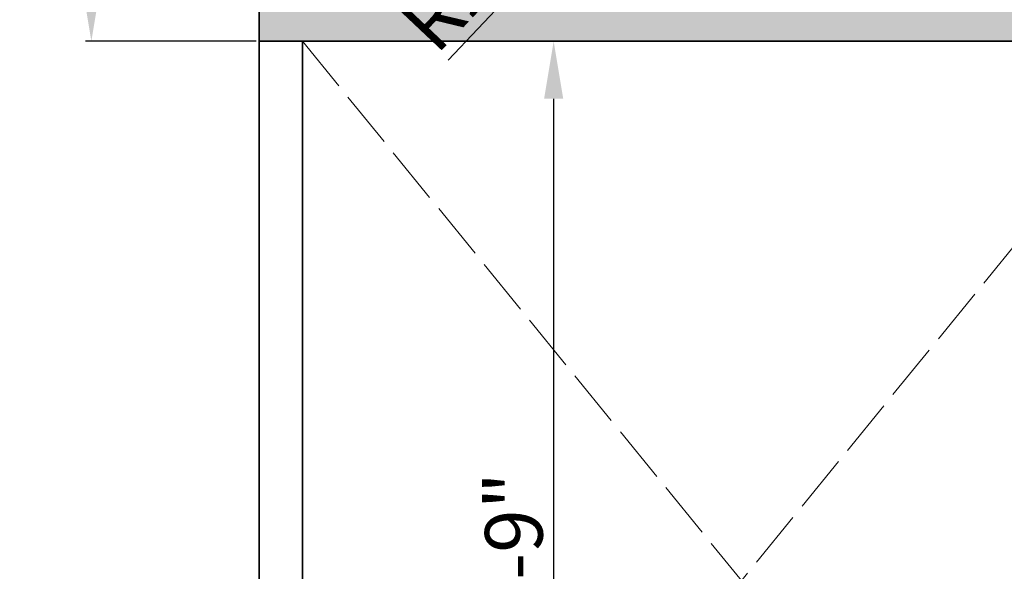
# Model space of a CAD drawing. Units: inches. Extents: x 2083 to 3317, y 1141 to 2115.
# Tile 83 of 256: x 2177 to 2382, y 1592 to 1707. Entities that reach past the tile are written whole.
import ezdxf

# ---------------------------------------------------------------- set-up
doc = ezdxf.new("R2010")
doc.units = ezdxf.units.IN
doc.linetypes.add('ACAD_ISO02W100', pattern=[15, 12, -3])
for name, color, linetype, lineweight in [('A-ANNO-DIMS', 2, 'Continuous', 18), ('A-FLOR-OPEN', 8, 'ACAD_ISO02W100', 13), ('A-WALL', 7, 'Continuous', 35)]:
    doc.layers.add(name, color=color, linetype=linetype, lineweight=lineweight)
doc.layers.add('A-WALL-PATT', color=251, linetype='Continuous', lineweight=13, true_color=0x636466)
doc.styles.get("Standard").update_dxf_attribs({"font": 'arial.ttf'})
doc.dimstyles.new('ISO-25', dxfattribs={"dimtxt": 12, "dimasz": 12, "dimexe": 1.25, "dimexo": 0.625, "dimtad": 1, "dimlunit": 3, "dimtxsty": 'Standard', "dimcen": 2.5, "dimadec": 0, "dimazin": 0, "dimtfac": 1, "dimtmove": 0, "dimatfit": 3, "dimfxl": 1, "dimarcsym": 0})

# ---------------------------------------------------------------- blocks, each defined once
blk = doc.blocks.new('*D14')
at = {"layer": 'A-ANNO-DIMS', "color": 0, "lineweight": -2, "transparency": 16777216}
for p, q in [((2226.33, 2020.76), (2190.73, 2020.76)), ((2191.98, 1714.76), (2191.98, 2008.76)), ((2226.33, 1702.76), (2190.73, 1702.76))]:
    blk.add_line(p, q, dxfattribs=at)
at = {"layer": 'A-ANNO-DIMS', "color": 0, "transparency": 16777216}
for points in [[(2189.98, 2008.76), (2193.98, 2008.76), (2191.98, 2020.76)], [(2189.98, 1714.76), (2193.98, 1714.76), (2191.98, 1702.76)]]:
    blk.add_solid(points, dxfattribs=at)
at = {"layer": 'Defpoints', "color": 0, "transparency": 16777216}
for p in [(2191.98, 2020.76), (2226.96, 2020.76), (2226.96, 1702.76)]:
    blk.add_point(p, dxfattribs=at)
at = {"layer": 'A-ANNO-DIMS', "color": 0, "transparency": 16777216, "insert": (2185.22, 1861.76), "char_height": 12, "attachment_point": 5, "rotation": 90}
blk.add_mtext('26\'-6"', dxfattribs=at)
blk = doc.blocks.new('*D64')
at = {"layer": 'A-ANNO-DIMS', "color": 0, "lineweight": -2, "transparency": 16777216}
for p, q in [((2236.58, 1702.76), (2289.56, 1702.76)), ((2288.31, 1690.76), (2288.31, 1489.76)), ((2236.58, 1477.76), (2289.56, 1477.76))]:
    blk.add_line(p, q, dxfattribs=at)
at = {"layer": 'A-ANNO-DIMS', "color": 0, "transparency": 16777216}
for points in [[(2286.31, 1690.76), (2290.31, 1690.76), (2288.31, 1702.76)], [(2286.31, 1489.76), (2290.31, 1489.76), (2288.31, 1477.76)]]:
    blk.add_solid(points, dxfattribs=at)
at = {"layer": 'Defpoints', "color": 0, "transparency": 16777216}
for p in [(2235.96, 1702.76), (2235.96, 1477.76), (2288.31, 1477.76)]:
    blk.add_point(p, dxfattribs=at)
at = {"layer": 'A-ANNO-DIMS', "color": 0, "transparency": 16777216, "insert": (2281.56, 1590.26), "char_height": 12, "attachment_point": 5, "rotation": 90}
blk.add_mtext('18\'-9"', dxfattribs=at)
blk = doc.blocks.new('*D69')
at = {"layer": 'A-ANNO-DIMS', "color": 0, "lineweight": -2, "transparency": 16777216}
for p, q in [((2355.6, 1793.35), (2332.67, 1769.07)), ((2266.34, 1698.84), (2324.43, 1760.34))]:
    blk.add_line(p, q, dxfattribs=at)
at = {"layer": 'A-ANNO-DIMS', "color": 0, "transparency": 16777216}
blk.add_solid([(2322.97, 1761.72), (2325.88, 1758.97), (2332.67, 1769.07)], dxfattribs=at)
at = {"layer": 'Defpoints', "color": 0, "transparency": 16777216}
for p in [(2355.6, 1793.35), (2332.67, 1769.07)]:
    blk.add_point(p, dxfattribs=at)
at = {"layer": 'A-ANNO-DIMS', "color": 0, "transparency": 16777216, "insert": (2286.3, 1729.92), "char_height": 12, "attachment_point": 5, "rotation": 46.6362}
blk.add_mtext('R2\'-9 1/2"', dxfattribs=at)

msp = doc.modelspace()

# ---------------------------------------------------------------- hatches: boundary and pattern name
at = {"layer": 'A-WALL-PATT'}
h = msp.add_hatch(color=256, dxfattribs=at)
h.dxf.hatch_style = 1
h.paths.add_polyline_path([(3126.96, 2020.761), (2748.96, 2020.761), (2604.96, 2020.761), (2226.96, 2020.761), (2226.96, 1702.761), (2466.96, 1702.761), (2466.96, 1582.761), (2418.96, 1582.761), (2418.96, 1477.761), (2226.96, 1477.761), (2226.96, 1263.261), (2544.96, 1263.261), (2544.96, 1411.761), (2604.96, 1411.761), (2685.96, 1411.761), (2685.96, 1420.761), (2604.96, 1420.761), (2604.96, 1573.761), (2604.96, 1702.761), (2604.96, 2011.761), (2748.96, 2011.761), (2748.96, 1702.761), (2862.96, 1702.761), (2862.96, 1621.761), (2871.96, 1621.761), (2871.96, 1702.761), (2883.96, 1702.761), (2883.96, 1706.939, -0.0264593), (2883.96, 1711.761), (2757.96, 1711.761), (2757.96, 1807.761), (2787.96, 1807.761), (2787.96, 1812.261), (2757.96, 1812.261), (2757.96, 2011.761), (2877.96, 2011.761), (2877.96, 1812.261), (2847.96, 1812.261), (2847.96, 1807.761), (2889.836, 1807.761), (2889.836, 1812.261), (2882.46, 1812.261), (2882.46, 2011.761), (3117.96, 2011.761), (3117.96, 1812.261), (2937.836, 1812.261), (2937.836, 1807.761), (2995.71, 1807.761), (2995.71, 1796.118), (3000.21, 1796.118), (3000.21, 1807.761), (3117.96, 1807.761), (3117.96, 1711.761), (3000.21, 1711.761), (3000.21, 1760.118), (2998.573, 1760.118, -0.020711), (2995.71, 1760.118), (2995.71, 1711.761), (2931.96, 1711.761), (2931.96, 1702.761), (3126.96, 1702.761)])
h.paths.add_polyline_path([(2471.46, 2011.761), (2471.46, 1810.011), (2462.717, 1810.011), (2462.717, 1805.511), (2505.96, 1805.511), (2505.96, 1810.011), (2475.96, 1810.011), (2475.96, 2011.761), (2595.96, 2011.761), (2595.96, 1810.011), (2565.96, 1810.011), (2565.96, 1805.511), (2595.96, 1805.511), (2595.96, 1711.761), (2235.96, 1711.761), (2235.96, 1805.511), (2353.71, 1805.511), (2353.71, 1796.054), (2358.21, 1796.054), (2358.21, 1805.511), (2414.717, 1805.511), (2414.717, 1810.011), (2235.96, 1810.011), (2235.96, 2011.761)], flags=16)
h.paths.add_polyline_path([(2270.205, 1994.61), (2270.205, 1970.61), (2246.205, 1970.61), (2246.205, 1994.61)], flags=0)
edge = h.paths.add_edge_path(flags=0)
edge.add_ellipse((2332.027, 1899.798), major_axis=(-3.043, 3.043), ratio=0.1682525, start_angle=-161.33217, end_angle=-156.30711, ccw=False)
edge.add_ellipse((2333.082, 1898.744), major_axis=(-1.055, 1.055), ratio=0.4535321, start_angle=-123.37102, end_angle=-94.15911)
edge = h.paths.add_edge_path(flags=0)
edge.add_ellipse((2332.027, 1968.876), major_axis=(3.043, 3.043), ratio=0.1682525, start_angle=18.66783, end_angle=23.69289)
edge.add_spline(control_points=[(2332.926, 1970.691), (2332.227, 1970.336), (2330.894, 1969.659), (2328.413, 1970.932), (2327.204, 1967.749), (2324.71, 1969.956), (2322.533, 1967.012), (2320.013, 1971.296), (2317.68, 1968.158), (2316.041, 1967.102), (2315.427, 1966.81)], knot_values=[0, 0, 0, 0, 2.2670587, 4.3245589, 6.6855835, 8.8786411, 11.121502, 14.300359, 17.7552837, 19.732645, 19.732645, 19.732645, 19.732645], degree=3, periodic=0)
edge.add_ellipse((2332.027, 1968.876), major_axis=(3.043, 3.043), ratio=0.1682525, start_angle=18.66783, end_angle=23.69289, ccw=False)
edge.add_ellipse((2333.082, 1969.931), major_axis=(1.055, 1.055), ratio=0.4535321, start_angle=56.62898, end_angle=85.84089, ccw=False)
edge = h.paths.add_edge_path(flags=0)
edge.add_spline(control_points=[(2296.428, 1967.988), (2293.628, 1965.336), (2287.704, 1959.727), (2299.744, 1949.996), (2294.533, 1935.669), (2290.573, 1920.604), (2293.394, 1909.974), (2296.185, 1904.967)], knot_values=[0.0991853, 0.0991853, 0.0991853, 0.0991853, 0.3453009, 0.6198217, 0.9826526, 1.3860932, 1.8105546, 1.8105546, 1.8105546, 1.8105546], degree=3, periodic=0)
edge.add_spline(control_points=[(2296.185, 1904.967), (2297.384, 1902.619), (2298.001, 1901.949), (2298.553, 1901.468)], knot_values=[0.0062457, 0.0062457, 0.0062457, 0.0062457, 0.0554759, 0.0554759, 0.0554759, 0.0554759], degree=3, periodic=0)
edge.add_spline(control_points=[(2298.553, 1901.468), (2297.259, 1900.923), (2295.225, 1900.232), (2293.06, 1900.614), (2292.101, 1900.788), (2292.09, 1900.791)], knot_values=[0.3128349, 0.3128349, 0.3128349, 0.3128349, 0.4017797, 0.4749867, 0.4759027, 0.4759027, 0.4759027, 0.4759027], degree=3, periodic=0)
edge.add_arc((2292.794, 1904.664), 3.937, 215.4209, 259.69818, ccw=False)
edge.add_spline(control_points=[(2289.585, 1902.382), (2289.477, 1902.535), (2289.368, 1902.688), (2289.261, 1902.841)], knot_values=[0.1028719, 0.1028719, 0.1028719, 0.1028719, 0.1168958, 0.1168958, 0.1168958, 0.1168958], degree=3, periodic=0)
edge.add_spline(control_points=[(2289.261, 1902.841), (2288.687, 1902.55), (2287.64, 1902.02), (2285.881, 1901.874), (2283.853, 1901.504), (2281.72, 1899.711), (2278.467, 1899.493), (2276.157, 1901.883), (2272.259, 1899.804), (2267.778, 1901.843), (2262.244, 1900.184), (2257.415, 1901.782), (2254.318, 1900.726), (2253.178, 1900.337)], knot_values=[0, 0, 0, 0, 1.9079767, 3.4771759, 5.261074, 7.9728515, 11.6802485, 13.7179214, 16.9395917, 22.789562, 27.5025027, 33.5952153, 37.1456181, 37.1456181, 37.1456181, 37.1456181], degree=3, periodic=0)
edge.add_line((2253.178, 1900.337), (2250.244, 1902.841))
edge.add_line((2250.244, 1902.841), (2250.244, 1965.833))
edge.add_line((2250.244, 1965.833), (2253.178, 1968.337))
edge.add_spline(control_points=[(2253.178, 1968.337), (2254.318, 1967.948), (2257.415, 1966.892), (2262.244, 1968.49), (2267.778, 1966.831), (2271.527, 1968.537), (2273.876, 1967.828), (2274.207, 1967.728)], knot_values=[0, 0, 0, 0, 0.0901802, 0.2449351, 0.3646438, 0.5132331, 0.5378548, 0.5378548, 0.5378548, 0.5378548], degree=3, periodic=0)
edge.add_arc((2274.353, 1963.793), 3.937, 72.05113, 92.12795, ccw=False)
edge.add_arc((2281.297, 1985.23), 18.596, 252.05113, 288.56572)
edge.add_arc((2292.317, 1956.029), 12.646, 71.02679, 113.77822, ccw=False)
edge = h.paths.add_edge_path(flags=0)
edge.add_spline(control_points=[(2274.899, 1951.856), (2275.066, 1951.617), (2275.233, 1951.377), (2275.398, 1951.136)], knot_values=[1.4099157, 1.4099157, 1.4099157, 1.4099157, 1.4315903, 1.4315903, 1.4315903, 1.4315903], degree=3, periodic=0)
edge.add_spline(control_points=[(2275.398, 1951.136), (2275.792, 1950.562), (2276.179, 1949.984), (2276.546, 1949.397)], knot_values=[1.3582378, 1.3582378, 1.3582378, 1.3582378, 1.4099157, 1.4099157, 1.4099157, 1.4099157], degree=3, periodic=0)
edge.add_line((2276.546, 1949.397), (2277.437, 1947.862))
edge.add_spline(control_points=[(2277.437, 1947.862), (2276.304, 1945.673), (2274.64, 1942.427), (2274.632, 1938.094), (2272.799, 1930.852), (2274.356, 1943.897), (2275.948, 1947.923), (2276.546, 1949.397)], knot_values=[0.0056315, 0.0056315, 0.0056315, 0.0056315, 0.1860139, 0.2660015, 0.3570872, 0.5963902, 0.7397317, 0.7397317, 0.7397317, 0.7397317], degree=3, periodic=0)
edge.add_spline(control_points=[(2276.546, 1949.397), (2276.179, 1949.984), (2275.792, 1950.562), (2275.398, 1951.136)], knot_values=[1.3582378, 1.3582378, 1.3582378, 1.3582378, 1.4099157, 1.4099157, 1.4099157, 1.4099157], degree=3, periodic=0)
edge.add_spline(control_points=[(2275.398, 1951.136), (2274.943, 1950.08), (2274.208, 1948.025), (2273.935, 1944.851), (2272.469, 1937.627), (2273.466, 1945.696), (2274.701, 1951.059), (2274.899, 1951.856)], knot_values=[0.1043639, 0.1043639, 0.1043639, 0.1043639, 0.1896363, 0.2696239, 0.3607096, 0.6000126, 0.6446217, 0.6446217, 0.6446217, 0.6446217], degree=3, periodic=0)
h.paths.add_polyline_path([(2269.168, 1963.128, -0.3575267), (2268.171, 1960.976, -0.0925607), (2268.171, 1939.436, -0.3575267), (2269.168, 1937.285, -0.3575267), (2267.016, 1938.282, -0.1647847), (2254.686, 1938.282, -0.3575267), (2252.534, 1937.285, -0.3575267), (2253.531, 1939.436, -0.0925607), (2253.531, 1960.976, -0.3575267), (2252.534, 1963.128, -0.3575267), (2254.686, 1962.131, -0.1647847), (2267.016, 1962.131, -0.3575267)], flags=0)
h.paths.add_polyline_path([(2248.874, 1967.802), (2248.874, 1957.028), (2249.458, 1957.028), (2249.458, 1911.647), (2248.874, 1911.647), (2248.874, 1900.873), (2246.512, 1900.873, 0.1973271), (2244.15, 1902.457), (2244.15, 1966.218, 0.1973271), (2246.512, 1967.802)], flags=0)
h.paths.add_polyline_path([(2269.168, 1931.389, -0.3575267), (2268.171, 1929.238, -0.0925607), (2268.171, 1907.698, -0.3575267), (2269.168, 1905.547, -0.3575267), (2267.016, 1906.544, -0.1647847), (2254.686, 1906.544, -0.3575267), (2252.534, 1905.547, -0.3575267), (2253.531, 1907.698, -0.0925607), (2253.531, 1929.238, -0.3575267), (2252.534, 1931.389, -0.3575267), (2254.686, 1930.392, -0.1647847), (2267.016, 1930.392, -0.3575267)], flags=0)
edge = h.paths.add_edge_path(flags=0)
edge.add_spline(control_points=[(2276.197, 1906.724), (2276.168, 1909.029), (2276.114, 1913.372), (2270.598, 1924.925), (2273.905, 1919.013), (2275.922, 1916.262), (2275.475, 1912.402), (2277.258, 1910.381), (2276.696, 1908.225), (2276.646, 1906.813), (2276.618, 1906.008)], knot_values=[0, 0, 0, 0, 8.6102597, 16.2212739, 18.8430575, 23.8048978, 27.4408283, 29.3561016, 31.2034776, 33.6506866, 33.6506866, 33.6506866, 33.6506866], degree=3, periodic=0)
edge.add_spline(control_points=[(2276.618, 1906.008), (2276.623, 1905.624), (2276.498, 1904.629), (2275.442, 1903.855), (2274.937, 1903.08), (2274.859, 1902.841)], knot_values=[0.1564884, 0.1564884, 0.1564884, 0.1564884, 0.1843975, 0.2313765, 0.2505985, 0.2505985, 0.2505985, 0.2505985], degree=3, periodic=0)
edge.add_line((2274.859, 1902.841), (2276.506, 1902.841))
edge.add_spline(control_points=[(2276.506, 1902.841), (2276.788, 1903.085), (2277.665, 1904.125), (2278.25, 1904.341), (2277.654, 1908.527), (2278.156, 1906.228), (2278.1, 1905.286), (2278.847, 1904.069), (2277.857, 1903.415), (2277.874, 1902.991), (2277.904, 1902.841)], knot_values=[0.0595743, 0.0595743, 0.0595743, 0.0595743, 0.0807529, 0.1037415, 0.1697201, 0.1760361, 0.2071372, 0.2404744, 0.2623409, 0.2736605, 0.2736605, 0.2736605, 0.2736605], degree=3, periodic=0)
edge.add_line((2277.904, 1902.841), (2280.03, 1902.841))
edge.add_spline(control_points=[(2280.03, 1902.841), (2279.888, 1903.088), (2279.499, 1903.982), (2280.152, 1905.939), (2278.104, 1909.658), (2279.762, 1907.185), (2280.328, 1904.875), (2280.485, 1903.49), (2281.463, 1903.249), (2281.758, 1902.936), (2281.834, 1902.841)], knot_values=[0.013856, 0.013856, 0.013856, 0.013856, 0.0348738, 0.0888667, 0.1078792, 0.1267378, 0.158714, 0.1937575, 0.2174868, 0.2267221, 0.2267221, 0.2267221, 0.2267221], degree=3, periodic=0)
edge.add_spline(control_points=[(2281.834, 1902.841), (2281.788, 1902.827), (2281.647, 1902.783), (2281.396, 1902.859), (2281.088, 1902.985), (2280.721, 1903.061), (2280.333, 1903.026), (2280.125, 1902.899), (2280.03, 1902.841)], knot_values=[0, 0, 0, 0, 0.1441304, 0.435517, 0.7492759, 1.1530457, 1.5483707, 1.878348, 1.878348, 1.878348, 1.878348], degree=3, periodic=0)
edge.add_line((2280.03, 1902.841), (2277.904, 1902.841))
edge.add_spline(control_points=[(2277.904, 1902.841), (2277.893, 1902.796), (2277.865, 1902.68), (2277.607, 1902.687), (2277.274, 1902.801), (2276.838, 1902.62), (2276.584, 1902.789), (2276.506, 1902.841)], knot_values=[0, 0, 0, 0, 0.1271885, 0.3261988, 0.6280094, 1.2435704, 1.5153306, 1.5153306, 1.5153306, 1.5153306], degree=3, periodic=0)
edge.add_line((2276.506, 1902.841), (2274.859, 1902.841))
edge.add_spline(control_points=[(2274.859, 1902.841), (2274.814, 1902.899), (2274.725, 1903.013), (2274.493, 1903.119), (2274.244, 1902.961), (2273.937, 1903.185), (2273.614, 1902.983), (2273.408, 1902.883), (2273.322, 1902.841)], knot_values=[0, 0, 0, 0, 0.2184302, 0.4369566, 0.6879766, 0.9903786, 1.3983955, 1.6918498, 1.6918498, 1.6918498, 1.6918498], degree=3, periodic=0)
edge.add_spline(control_points=[(2273.322, 1902.841), (2273.617, 1903.446), (2274.274, 1904.538), (2276.027, 1904.574), (2276.207, 1906.584), (2276.197, 1906.724)], knot_values=[0.0122268, 0.0122268, 0.0122268, 0.0122268, 0.0594721, 0.1062177, 0.134458, 0.134458, 0.134458, 0.134458], degree=3, periodic=0)
h.paths.add_polyline_path([(2270.776, 1897.79), (2270.776, 1873.79), (2246.776, 1873.79), (2246.776, 1897.79)], flags=0)
h.paths.add_polyline_path([(2353.71, 1760.005), (2353.71, 1760.054), (2358.21, 1760.054, -0.033729)], flags=0)
h.paths.add_polyline_path([(2321.819, 1737.529), (2341.995, 1737.529, -0.4142136), (2343.203, 1736.321), (2343.203, 1721.021, -0.4142136), (2341.995, 1719.813), (2321.819, 1719.813, -0.4142136), (2320.611, 1721.021), (2320.611, 1736.321, -0.4142136)], flags=0)
h.paths.add_polyline_path([(2324.235, 1736.321), (2339.579, 1736.321, -0.4142136), (2341.995, 1733.905), (2341.995, 1725.45, -0.4142136), (2339.579, 1723.034), (2333.681, 1723.034), (2333.845, 1722.045, -0.8706461), (2335.425, 1721.826, -0.767327), (2333.923, 1721.423), (2331.291, 1721.423, -0.767327), (2329.788, 1721.826, -0.8706461), (2331.368, 1722.045), (2331.533, 1723.034), (2324.235, 1723.034, -0.4142136), (2321.819, 1725.45), (2321.819, 1733.905, -0.4142136)], flags=0)
h.paths.add_polyline_path([(2570.484, 1928.615), (2589.684, 1928.615), (2590.169, 1928.615), (2590.169, 1904.993), (2570.484, 1904.993)], flags=0)
h.paths.add_polyline_path([(2574.447, 1927.264, -1), (2572.829, 1927.264, -1)], flags=0)
h.paths.add_polyline_path([(2573.09, 1926.941), (2573.925, 1927.776), (2574.148, 1927.553), (2573.313, 1926.718)], flags=0)
h.paths.add_polyline_path([(2578.779, 1919.73, -1), (2571.592, 1919.73, -1)], flags=0)
h.paths.add_polyline_path([(2578.385, 1919.73, -1), (2571.985, 1919.73, -1)], flags=0)
h.paths.add_polyline_path([(2331.596, 1729.476, -1), (2333.618, 1729.476, -1)], flags=0)
h.paths.add_polyline_path([(2578.034, 1927.264, -1), (2576.416, 1927.264, -1)], flags=0)
h.paths.add_polyline_path([(2576.689, 1927.531), (2576.912, 1927.754), (2577.747, 1926.919), (2577.524, 1926.696)], flags=0)
h.paths.add_polyline_path([(2578.139, 1909.86, -1), (2572.232, 1909.86, -1)], flags=0)
h.paths.add_polyline_path([(2577.745, 1909.86, -1), (2572.625, 1909.86, -1)], flags=0)
h.paths.add_polyline_path([(2583.798, 1927.264, -1), (2582.179, 1927.264, -1)], flags=0)
h.paths.add_polyline_path([(2582.719, 1927.754), (2583.554, 1926.919), (2583.331, 1926.696), (2582.496, 1927.531)], flags=0)
h.paths.add_polyline_path([(2582.496, 1927.531), (2582.719, 1927.754), (2583.554, 1926.919), (2583.331, 1926.696)], flags=0)
h.paths.add_polyline_path([(2587.739, 1920.53, -1), (2581.832, 1920.53, -1)], flags=0)
h.paths.add_polyline_path([(2587.345, 1920.53, -1), (2582.225, 1920.53, -1)], flags=0)
h.paths.add_polyline_path([(2587.385, 1927.264, -1), (2585.766, 1927.264, -1)], flags=0)
h.paths.add_polyline_path([(2586.082, 1926.98), (2586.917, 1927.815), (2587.14, 1927.593), (2586.305, 1926.758)], flags=0)
h.paths.add_polyline_path([(2588.379, 1910.66, -1), (2581.192, 1910.66, -1)], flags=0)
h.paths.add_polyline_path([(2587.985, 1910.66, -1), (2581.585, 1910.66, -1)], flags=0)
h.paths.add_polyline_path([(2417.168, 1729.478), (2437.344, 1729.478, -0.4142136), (2438.552, 1728.27), (2438.552, 1712.969, -0.4142136), (2437.344, 1711.761), (2417.168, 1711.761, -0.4142136), (2415.96, 1712.969), (2415.96, 1728.27, -0.4142136)], flags=0)
h.paths.add_polyline_path([(2419.584, 1728.27), (2434.928, 1728.27, -0.4142136), (2437.344, 1725.854), (2437.344, 1717.398, -0.4142136), (2434.928, 1714.983), (2429.029, 1714.983), (2429.194, 1713.994, -0.8706461), (2430.774, 1713.775, -0.767327), (2429.271, 1713.372), (2426.64, 1713.372, -0.767327), (2425.137, 1713.775, -0.8706461), (2426.717, 1713.994), (2426.882, 1714.983), (2419.584, 1714.983, -0.4142136), (2417.168, 1717.398), (2417.168, 1725.854, -0.4142136)], flags=0)
h.paths.add_polyline_path([(2419.584, 1728.27), (2434.928, 1728.27, -0.4142136), (2437.344, 1725.854), (2437.344, 1717.398, -0.4142136), (2434.928, 1714.983), (2429.029, 1714.983), (2428.358, 1719.009), (2427.553, 1719.009), (2426.882, 1714.983), (2419.584, 1714.983, -0.4142136), (2417.168, 1717.398), (2417.168, 1725.854, -0.4142136)], flags=0)
h.paths.add_polyline_path([(2426.944, 1721.425, -1), (2428.967, 1721.425, -1)], flags=0)
h.paths.add_polyline_path([(2475.96, 1702.761), (2595.96, 1702.761), (2595.96, 1582.761), (2475.96, 1582.761)], flags=16)
h.paths.add_polyline_path([(2427.96, 1573.761), (2595.96, 1573.761), (2595.96, 1468.761), (2595.96, 1420.761), (2384.46, 1420.761), (2384.46, 1468.761), (2427.96, 1468.761)], flags=16)
h.paths.add_polyline_path([(2379.96, 1468.761), (2379.96, 1420.761), (2235.96, 1420.761), (2235.96, 1468.761)], flags=16)
h.paths.add_polyline_path([(2317.816, 1466.696), (2337.992, 1466.696, -0.4142136), (2339.2, 1465.488), (2339.2, 1450.187, -0.4142136), (2337.992, 1448.979), (2317.816, 1448.979, -0.4142136), (2316.608, 1450.187), (2316.608, 1465.488, -0.4142136)], flags=0)
h.paths.add_polyline_path([(2320.232, 1465.488), (2335.576, 1465.488, -0.4142136), (2337.992, 1463.072), (2337.992, 1454.616, -0.4142136), (2335.576, 1452.2), (2329.677, 1452.2), (2329.842, 1451.212, -0.8706461), (2331.422, 1450.992, -0.767327), (2329.92, 1450.59), (2327.288, 1450.59, -0.767327), (2325.785, 1450.992, -0.8706461), (2327.365, 1451.212), (2327.53, 1452.2), (2320.232, 1452.2, -0.4142136), (2317.816, 1454.616), (2317.816, 1463.072, -0.4142136)], flags=0)
h.paths.add_polyline_path([(2320.232, 1465.488), (2335.576, 1465.488, -0.4142136), (2337.992, 1463.072), (2337.992, 1454.616, -0.4142136), (2335.576, 1452.2), (2329.677, 1452.2), (2329.006, 1456.227), (2328.201, 1456.227), (2327.53, 1452.2), (2320.232, 1452.2, -0.4142136), (2317.816, 1454.616), (2317.816, 1463.072, -0.4142136)], flags=0)
h.paths.add_polyline_path([(2327.593, 1458.643, -1), (2329.615, 1458.643, -1)], flags=0)
h.paths.add_polyline_path([(2244.412, 1433.34), (2241.921, 1433.34, -0.4142136), (2240.018, 1435.244), (2240.018, 1440.953, -0.4142105), (2241.921, 1442.856), (2244.412, 1442.856, -1.9764724)], flags=0)
h.paths.add_polyline_path([(2245.357, 1434.398, -0.4142136), (2245.357, 1441.799, -2.1440985)], flags=0)
h.paths.add_polyline_path([(2535.96, 1416.261), (2535.96, 1272.261), (2235.96, 1272.261), (2235.96, 1416.261)], flags=16)
h.paths.add_polyline_path([(2260.12, 1384.293), (2260.12, 1362.039), (2237.865, 1362.039), (2237.865, 1384.293)], flags=0)
edge = h.paths.add_edge_path(flags=0)
edge.add_line((2318.252, 1362.093), (2318.146, 1362.001))
edge.add_ellipse((2317.445, 1360.431), major_axis=(2.822, 2.822), ratio=0.1682525, start_angle=18.66783, end_angle=20.94813, ccw=False)
edge.add_ellipse((2318.423, 1361.409), major_axis=(0.978, 0.978), ratio=0.4535321, start_angle=56.62898, end_angle=70.2262, ccw=False)
edge = h.paths.add_edge_path(flags=0)
edge.add_line((2319.107, 1295.571), (2319.015, 1295.677))
edge.add_ellipse((2317.445, 1296.378), major_axis=(-2.822, 2.822), ratio=0.1682525, start_angle=-161.33217, end_angle=-159.05187, ccw=False)
edge.add_ellipse((2318.423, 1295.4), major_axis=(-0.978, 0.978), ratio=0.4535321, start_angle=-123.37102, end_angle=-109.7738)
edge = h.paths.add_edge_path(flags=0)
edge.add_spline(control_points=[(2284.21, 1301.17), (2284.581, 1300.445), (2284.891, 1299.892), (2285.16, 1299.461)], knot_values=[0.0390658, 0.0390658, 0.0390658, 0.0390658, 0.0554759, 0.0554759, 0.0554759, 0.0554759], degree=3, periodic=0)
edge.add_line((2285.16, 1299.461), (2284.21, 1301.17))
edge = h.paths.add_edge_path(flags=0)
edge.add_line((2280.412, 1297.298), (2283.37, 1297.036))
edge.add_line((2283.37, 1297.036), (2286.406, 1297.926))
edge.add_spline(control_points=[(2286.406, 1297.926), (2285.305, 1297.463), (2284.345, 1297.129), (2283.37, 1297.036)], knot_values=[0.3943688, 0.3943688, 0.3943688, 0.3943688, 0.4759027, 0.4759027, 0.4759027, 0.4759027], degree=3, periodic=0)
edge.add_spline(control_points=[(2283.37, 1297.036), (2283.281, 1297.028), (2282.316, 1296.957), (2281.313, 1297.134), (2280.423, 1297.296), (2280.412, 1297.298)], knot_values=[0.3128349, 0.3128349, 0.3128349, 0.3128349, 0.3202458, 0.3934528, 0.3943688, 0.3943688, 0.3943688, 0.3943688], degree=3, periodic=0)
edge = h.paths.add_edge_path(flags=0)
edge.add_line((2284.436, 1359.607), (2280.446, 1355.328))
edge.add_line((2280.446, 1355.328), (2279.58, 1351.018))
edge.add_line((2279.58, 1351.018), (2282.413, 1346.58))
edge.add_spline(control_points=[(2282.413, 1346.58), (2283.153, 1345.589), (2284.253, 1344.029), (2284.801, 1342.387), (2284.935, 1341.806)], knot_values=[1.2400982, 1.2400982, 1.2400982, 1.2400982, 1.3328922, 1.3827123, 1.3827123, 1.3827123, 1.3827123], degree=3, periodic=0)
edge.add_spline(control_points=[(2284.935, 1341.806), (2285.319, 1340.141), (2285.233, 1338.409), (2284.91, 1336.654)], knot_values=[1.0974841, 1.0974841, 1.0974841, 1.0974841, 1.2400982, 1.2400982, 1.2400982, 1.2400982], degree=3, periodic=0)
edge.add_spline(control_points=[(2284.91, 1336.654), (2284.587, 1334.899), (2284.027, 1333.12), (2283.463, 1331.361)], knot_values=[0.9548699, 0.9548699, 0.9548699, 0.9548699, 1.0974841, 1.0974841, 1.0974841, 1.0974841], degree=3, periodic=0)
edge.add_line((2283.463, 1331.361), (2281.89, 1326.153))
edge.add_line((2281.89, 1326.153), (2280.756, 1321.056))
edge.add_line((2280.756, 1321.056), (2280.299, 1316.002))
edge.add_line((2280.299, 1316.002), (2280.716, 1310.95))
edge.add_line((2280.716, 1310.95), (2282.028, 1305.972))
edge.add_line((2282.028, 1305.972), (2284.21, 1301.17))
edge.add_spline(control_points=[(2284.21, 1301.17), (2283.341, 1302.73), (2282.612, 1304.336), (2282.028, 1305.972)], knot_values=[0.0991853, 0.0991853, 0.0991853, 0.0991853, 0.2417994, 0.2417994, 0.2417994, 0.2417994], degree=3, periodic=0)
edge.add_spline(control_points=[(2282.028, 1305.972), (2281.444, 1307.608), (2281.005, 1309.273), (2280.716, 1310.95)], knot_values=[0.2417994, 0.2417994, 0.2417994, 0.2417994, 0.3844135, 0.3844135, 0.3844135, 0.3844135], degree=3, periodic=0)
edge.add_spline(control_points=[(2280.716, 1310.95), (2280.433, 1312.588), (2280.289, 1314.277), (2280.299, 1315.962), (2280.299, 1316.002)], knot_values=[0.3844135, 0.3844135, 0.3844135, 0.3844135, 0.5236467, 0.5270276, 0.5270276, 0.5270276, 0.5270276], degree=3, periodic=0)
edge.add_spline(control_points=[(2280.299, 1316.002), (2280.312, 1317.687), (2280.478, 1319.368), (2280.756, 1321.056)], knot_values=[0.5270276, 0.5270276, 0.5270276, 0.5270276, 0.6696417, 0.6696417, 0.6696417, 0.6696417], degree=3, periodic=0)
edge.add_spline(control_points=[(2280.756, 1321.056), (2281.035, 1322.744), (2281.426, 1324.44), (2281.89, 1326.153)], knot_values=[0.6696417, 0.6696417, 0.6696417, 0.6696417, 0.8122558, 0.8122558, 0.8122558, 0.8122558], degree=3, periodic=0)
edge.add_spline(control_points=[(2281.89, 1326.153), (2282.264, 1327.533), (2282.788, 1329.262), (2283.353, 1331.018), (2283.463, 1331.361)], knot_values=[0.8122558, 0.8122558, 0.8122558, 0.8122558, 0.9270873, 0.9548699, 0.9548699, 0.9548699, 0.9548699], degree=3, periodic=0)
edge.add_line((2283.463, 1331.361), (2284.91, 1336.654))
edge.add_line((2284.91, 1336.654), (2284.935, 1341.806))
edge.add_line((2284.935, 1341.806), (2282.413, 1346.58))
edge.add_spline(control_points=[(2282.413, 1346.58), (2281.275, 1348.104), (2280.078, 1349.57), (2279.58, 1351.018)], knot_values=[1.3827123, 1.3827123, 1.3827123, 1.3827123, 1.5253264, 1.5253264, 1.5253264, 1.5253264], degree=3, periodic=0)
edge.add_spline(control_points=[(2279.58, 1351.018), (2279.443, 1351.415), (2279.136, 1352.857), (2279.735, 1354.29), (2280.446, 1355.328)], knot_values=[1.5253264, 1.5253264, 1.5253264, 1.5253264, 1.564439, 1.6679405, 1.6679405, 1.6679405, 1.6679405], degree=3, periodic=0)
edge.add_spline(control_points=[(2280.446, 1355.328), (2281.426, 1356.758), (2282.931, 1358.183), (2284.436, 1359.607)], knot_values=[1.6679405, 1.6679405, 1.6679405, 1.6679405, 1.8105546, 1.8105546, 1.8105546, 1.8105546], degree=3, periodic=0)
edge.add_arc((2280.623, 1348.518), 11.726, 71.02679, 113.77822)
edge.add_arc((2270.405, 1375.595), 17.244, 252.05113, 288.56572, ccw=False)
edge.add_arc((2263.966, 1355.718), 3.651, 72.05113, 92.12795)
edge.add_arc((2263.966, 1355.718), 3.651, 92.12795, 177.98513)
edge.add_spline(control_points=[(2260.318, 1355.846), (2260.26, 1354.221), (2260.551, 1350.187), (2262.999, 1346.766), (2264.473, 1344.649)], knot_values=[1.4315903, 1.4315903, 1.4315903, 1.4315903, 1.5641438, 1.7706953, 1.7706953, 1.7706953, 1.7706953], degree=3, periodic=0)
edge.add_line((2264.473, 1344.649), (2264.936, 1343.983))
edge.add_spline(control_points=[(2263.801, 1340.248), (2263.843, 1340.514), (2264.067, 1341.756), (2264.513, 1343.002), (2264.935, 1343.981)], knot_values=[0.5365702, 0.5365702, 0.5365702, 0.5365702, 0.5593494, 0.6446217, 0.6446217, 0.6446217, 0.6446217], degree=3, periodic=0)
edge.add_spline(control_points=[(2264.935, 1343.981), (2265.118, 1343.715), (2265.299, 1343.448), (2265.477, 1343.179)], knot_values=[1.3840767, 1.3840767, 1.3840767, 1.3840767, 1.4099157, 1.4099157, 1.4099157, 1.4099157], degree=3, periodic=0)
edge.add_spline(control_points=[(2265.477, 1343.179), (2265.655, 1342.911), (2265.829, 1342.641), (2265.999, 1342.369)], knot_values=[1.3582378, 1.3582378, 1.3582378, 1.3582378, 1.3840767, 1.3840767, 1.3840767, 1.3840767], degree=3, periodic=0)
edge.add_line((2265.999, 1342.369), (2266.826, 1340.946))
edge.add_spline(control_points=[(2266.826, 1340.946), (2268.894, 1337.09), (2271.398, 1325.843), (2270.516, 1310.569), (2275.919, 1301.861), (2277.79, 1299.199)], knot_values=[0.1168958, 0.1168958, 0.1168958, 0.1168958, 0.4729873, 1.0509689, 1.3137934, 1.3137934, 1.3137934, 1.3137934], degree=3, periodic=0)
edge.add_spline(control_points=[(2277.79, 1299.199), (2277.839, 1299.128), (2277.889, 1299.057), (2277.94, 1298.987)], knot_values=[0.1098839, 0.1098839, 0.1098839, 0.1098839, 0.1168958, 0.1168958, 0.1168958, 0.1168958], degree=3, periodic=0)
edge.add_line((2277.94, 1298.987), (2277.789, 1299.199))
edge.add_spline(control_points=[(2277.789, 1299.199), (2277.257, 1298.929), (2276.286, 1298.438), (2275.039, 1298.334), (2274.383, 1298.239), (2274.215, 1298.209)], knot_values=[33.1218702, 33.1218702, 33.1218702, 33.1218702, 35.0290557, 36.5982549, 37.1448269, 37.1448269, 37.1448269, 37.1448269], degree=3, periodic=0)
edge.add_line((2274.215, 1298.209), (2273.073, 1297.893))
edge.add_spline(control_points=[(2273.073, 1297.893), (2272.323, 1297.58), (2271.039, 1296.511), (2269.248, 1296.226), (2268.423, 1296.375)], knot_values=[26.5325843, 26.5325843, 26.5325843, 26.5325843, 29.198919, 31.8391012, 31.8391012, 31.8391012, 31.8391012], degree=3, periodic=0)
edge.add_line((2268.423, 1296.375), (2263.879, 1297.458))
edge.add_spline(control_points=[(2263.879, 1297.458), (2263.556, 1297.359), (2261.86, 1296.839), (2260.239, 1297.282), (2258.933, 1297.516)], knot_values=[15.9195506, 15.9195506, 15.9195506, 15.9195506, 16.9395917, 21.2260675, 21.2260675, 21.2260675, 21.2260675], degree=3, periodic=0)
edge.add_line((2258.933, 1297.516), (2254.055, 1297.329))
edge.add_spline(control_points=[(2254.055, 1297.329), (2253.756, 1297.296), (2252.114, 1297.165), (2250.462, 1297.544), (2249.13, 1297.668)], knot_values=[5.3065169, 5.3065169, 5.3065169, 5.3065169, 6.2764352, 10.6130337, 10.6130337, 10.6130337, 10.6130337], degree=3, periodic=0)
edge.add_line((2249.13, 1297.668), (2244.332, 1296.878))
edge.add_line((2244.332, 1296.878), (2241.611, 1299.199))
edge.add_line((2241.611, 1299.199), (2241.611, 1357.609))
edge.add_line((2241.611, 1357.609), (2244.332, 1359.931))
edge.add_line((2244.332, 1359.931), (2252.729, 1359.543))
edge.add_spline(control_points=[(2252.729, 1359.543), (2252.871, 1359.546), (2253.306, 1359.548), (2253.74, 1359.514), (2254.032, 1359.482)], knot_values=[0.233291, 0.233291, 0.233291, 0.233291, 0.2449351, 0.2689274, 0.2689274, 0.2689274, 0.2689274], degree=3, periodic=0)
edge.add_line((2254.032, 1359.482), (2259.587, 1359.416))
edge.add_spline(control_points=[(2259.587, 1359.416), (2260.677, 1359.629), (2262.073, 1359.897), (2263.524, 1359.459), (2263.83, 1359.366)], knot_values=[0.4225164, 0.4225164, 0.4225164, 0.4225164, 0.5132331, 0.5378548, 0.5378548, 0.5378548, 0.5378548], degree=3, periodic=0)
edge.add_arc((2263.966, 1355.718), 3.651, 72.05113, 92.12795, ccw=False)
edge.add_arc((2270.405, 1375.595), 17.244, 252.05113, 288.56572)
edge.add_arc((2280.623, 1348.518), 11.726, 71.02679, 113.77822, ccw=False)
h.paths.add_polyline_path([(2240.341, 1359.435), (2240.341, 1349.444), (2240.882, 1349.444), (2240.882, 1307.365), (2240.341, 1307.365), (2240.341, 1297.374), (2238.15, 1297.374, 0.1973271), (2235.96, 1298.843), (2235.96, 1357.966, 0.1973271), (2238.15, 1359.435)], flags=0)
h.paths.add_polyline_path([(2259.158, 1355.101, -0.3575267), (2258.233, 1353.106, -0.0925607), (2258.233, 1333.133, -0.3575267), (2259.158, 1331.138, -0.3575267), (2257.163, 1332.062, -0.1647847), (2245.729, 1332.062, -0.3575267), (2243.735, 1331.138, -0.3575267), (2244.659, 1333.133, -0.0925607), (2244.659, 1353.106, -0.3575267), (2243.735, 1355.101, -0.3575267), (2245.729, 1354.176, -0.1647847), (2257.163, 1354.176, -0.3575267)], flags=0)
edge = h.paths.add_edge_path(flags=0)
edge.add_line((2265.999, 1342.369), (2266.826, 1340.946))
edge.add_line((2266.826, 1340.946), (2265.308, 1337.814))
edge.add_line((2265.308, 1337.814), (2264.358, 1334.653))
edge.add_line((2264.358, 1334.653), (2264.262, 1333.8))
edge.add_spline(control_points=[(2264.262, 1333.8), (2264.208, 1333.187), (2264.162, 1332.366), (2264.007, 1331.414), (2263.969, 1331.202)], knot_values=[0.4644442, 0.4644442, 0.4644442, 0.4644442, 0.5166905, 0.5316081, 0.5316081, 0.5316081, 0.5316081], degree=3, periodic=0)
edge.add_spline(control_points=[(2263.969, 1331.202), (2263.775, 1330.119), (2263.424, 1328.791), (2263.257, 1328.531), (2263.234, 1328.515)], knot_values=[0.3726816, 0.3726816, 0.3726816, 0.3726816, 0.4488497, 0.4644442, 0.4644442, 0.4644442, 0.4644442], degree=3, periodic=0)
edge.add_spline(control_points=[(2263.234, 1328.515), (2263.096, 1328.42), (2263.131, 1329.301), (2263.275, 1330.616)], knot_values=[0.2809191, 0.2809191, 0.2809191, 0.2809191, 0.3726816, 0.3726816, 0.3726816, 0.3726816], degree=3, periodic=0)
edge.add_spline(control_points=[(2263.275, 1330.616), (2263.419, 1331.93), (2263.672, 1333.677), (2263.97, 1335.315)], knot_values=[0.1891566, 0.1891566, 0.1891566, 0.1891566, 0.2809191, 0.2809191, 0.2809191, 0.2809191], degree=3, periodic=0)
edge.add_spline(control_points=[(2263.97, 1335.315), (2264.1, 1336.032), (2264.419, 1337.622), (2264.755, 1338.864), (2264.947, 1339.491)], knot_values=[0.097394, 0.097394, 0.097394, 0.097394, 0.1375775, 0.1891566, 0.1891566, 0.1891566, 0.1891566], degree=3, periodic=0)
edge.add_spline(control_points=[(2264.947, 1339.491), (2265.29, 1340.606), (2265.644, 1341.494), (2265.999, 1342.369)], knot_values=[0.0056315, 0.0056315, 0.0056315, 0.0056315, 0.097394, 0.097394, 0.097394, 0.097394], degree=3, periodic=0)
h.paths.add_polyline_path([(2259.158, 1325.671, -0.3575267), (2258.233, 1323.676, -0.0925607), (2258.233, 1303.703, -0.3575267), (2259.158, 1301.708, -0.3575267), (2257.163, 1302.633, -0.1647847), (2245.729, 1302.633, -0.3575267), (2243.735, 1301.708, -0.3575267), (2244.659, 1303.703, -0.0925607), (2244.659, 1323.676, -0.3575267), (2243.735, 1325.671, -0.3575267), (2245.729, 1324.747, -0.1647847), (2257.163, 1324.747, -0.3575267)], flags=0)
edge = h.paths.add_edge_path(flags=0)
edge.add_spline(control_points=[(2261.709, 1317.311), (2261.679, 1317.418), (2261.762, 1317.389), (2262.491, 1316.09), (2262.962, 1315.301)], knot_values=[14.9558607, 14.9558607, 14.9558607, 14.9558607, 16.2212739, 18.6948259, 18.6948259, 18.6948259, 18.6948259], degree=3, periodic=0)
edge.add_spline(control_points=[(2262.962, 1315.301), (2262.99, 1315.254), (2263.702, 1314.067), (2264.349, 1313.127), (2264.73, 1312.164)], knot_values=[18.6948259, 18.6948259, 18.6948259, 18.6948259, 18.8430575, 22.433791, 22.433791, 22.433791, 22.433791], degree=3, periodic=0)
edge.add_spline(control_points=[(2264.73, 1312.164), (2264.876, 1311.796), (2265.177, 1310.77), (2265.143, 1309.559), (2265.248, 1308.824)], knot_values=[22.433791, 22.433791, 22.433791, 22.433791, 23.8048978, 26.1727562, 26.1727562, 26.1727562, 26.1727562], degree=3, periodic=0)
edge.add_line((2265.248, 1308.824), (2265.851, 1307.172))
edge.add_spline(control_points=[(2265.851, 1307.172), (2266.065, 1306.822), (2266.384, 1306.332), (2266.424, 1305.781), (2266.42, 1305.611)], knot_values=[28.0625624, 28.0625624, 28.0625624, 28.0625624, 29.3561016, 29.9117214, 29.9117214, 29.9117214, 29.9117214], degree=3, periodic=0)
edge.add_spline(control_points=[(2266.42, 1305.611), (2266.416, 1305.433), (2266.394, 1305.25), (2266.365, 1305.066)], knot_values=[29.9117214, 29.9117214, 29.9117214, 29.9117214, 30.4978371, 30.4978371, 30.4978371, 30.4978371], degree=3, periodic=0)
edge.add_line((2266.365, 1305.066), (2266.066, 1302.136))
edge.add_spline(control_points=[(2266.066, 1302.136), (2266.071, 1301.78), (2265.998, 1301.2), (2265.663, 1300.759), (2265.509, 1300.586)], knot_values=[0.1564884, 0.1564884, 0.1564884, 0.1564884, 0.1843975, 0.2035434, 0.2035434, 0.2035434, 0.2035434], degree=3, periodic=0)
edge.add_line((2265.509, 1300.586), (2264.435, 1299.199))
edge.add_line((2264.435, 1299.199), (2265.962, 1299.199))
edge.add_line((2265.962, 1299.199), (2267.336, 1301.175))
edge.add_line((2267.336, 1301.175), (2267.312, 1301.986))
edge.add_spline(control_points=[(2267.312, 1301.986), (2267.261, 1302.862), (2267.16, 1303.737), (2267.271, 1303.326)], knot_values=[0.1262286, 0.1262286, 0.1262286, 0.1262286, 0.1666174, 0.1666174, 0.1666174, 0.1666174], degree=3, periodic=0)
edge.add_spline(control_points=[(2267.271, 1303.326), (2267.28, 1303.294), (2267.31, 1303.175), (2267.373, 1302.884), (2267.406, 1302.683), (2267.418, 1302.601)], knot_values=[0.1666174, 0.1666174, 0.1666174, 0.1666174, 0.1697201, 0.1760361, 0.1807647, 0.1807647, 0.1807647, 0.1807647], degree=3, periodic=0)
edge.add_spline(control_points=[(2267.744, 1300.988), (2267.688, 1301.151), (2267.481, 1301.657), (2267.484, 1302.145), (2267.418, 1302.601)], knot_values=[0.1807647, 0.1807647, 0.1807647, 0.1807647, 0.1937665, 0.2201389, 0.2201389, 0.2201389, 0.2201389], degree=3, periodic=0)
edge.add_line((2267.418, 1302.601), (2267.744, 1300.988))
edge.add_spline(control_points=[(2267.744, 1300.988), (2267.832, 1300.732), (2267.932, 1300.31), (2267.555, 1299.975), (2267.429, 1299.829)], knot_values=[0.2201389, 0.2201389, 0.2201389, 0.2201389, 0.2404744, 0.2548903, 0.2548903, 0.2548903, 0.2548903], degree=3, periodic=0)
edge.add_line((2267.429, 1299.829), (2267.258, 1299.199))
edge.add_line((2267.258, 1299.199), (2269.23, 1299.199))
edge.add_spline(control_points=[(2269.23, 1299.199), (2269.099, 1299.429), (2268.843, 1300.016), (2269.012, 1300.916), (2268.947, 1301.661)], knot_values=[0.013856, 0.013856, 0.013856, 0.013856, 0.0348738, 0.0670726, 0.0670726, 0.0670726, 0.0670726], degree=3, periodic=0)
edge.add_line((2268.947, 1301.661), (2268.432, 1303.603))
edge.add_spline(control_points=[(2268.432, 1303.603), (2268.176, 1304.192), (2267.596, 1305.251), (2268.041, 1304.623), (2268.251, 1304.282)], knot_values=[0.0901547, 0.0901547, 0.0901547, 0.0901547, 0.1078792, 0.1202891, 0.1202891, 0.1202891, 0.1202891], degree=3, periodic=0)
edge.add_spline(control_points=[(2268.251, 1304.282), (2268.361, 1304.105), (2269.058, 1302.918), (2269.383, 1301.59), (2269.521, 1300.776), (2269.575, 1300.556)], knot_values=[0.1202891, 0.1202891, 0.1202891, 0.1202891, 0.1267378, 0.158714, 0.1735056, 0.1735056, 0.1735056, 0.1735056], degree=3, periodic=0)
edge.add_line((2269.575, 1300.556), (2270.686, 1299.421))
edge.add_spline(control_points=[(2270.686, 1299.421), (2270.767, 1299.357), (2270.838, 1299.281), (2270.903, 1299.199)], knot_values=[0.2181597, 0.2181597, 0.2181597, 0.2181597, 0.2267221, 0.2267221, 0.2267221, 0.2267221], degree=3, periodic=0)
edge.add_line((2270.937, 1299.193), (2270.903, 1299.199))
edge.add_spline(control_points=[(2270.903, 1299.199), (2270.86, 1299.186), (2270.73, 1299.146), (2270.496, 1299.216), (2270.272, 1299.308), (2270.121, 1299.348), (2270.063, 1299.36)], knot_values=[0.939174, 0.939174, 0.939174, 0.939174, 1.0833044, 1.3746911, 1.6884499, 1.878348, 1.878348, 1.878348, 1.878348], degree=3, periodic=0)
edge.add_line((2270.063, 1299.36), (2269.23, 1299.199))
edge.add_line((2269.23, 1299.199), (2267.258, 1299.199))
edge.add_spline(control_points=[(2267.258, 1299.199), (2267.248, 1299.157), (2267.223, 1299.05), (2266.984, 1299.057), (2266.809, 1299.116), (2266.677, 1299.109), (2266.637, 1299.105)], knot_values=[0.7576653, 0.7576653, 0.7576653, 0.7576653, 0.8848538, 1.0838641, 1.3856747, 1.5153306, 1.5153306, 1.5153306, 1.5153306], degree=3, periodic=0)
edge.add_spline(control_points=[(2266.637, 1299.105), (2266.485, 1299.089), (2266.236, 1299.017), (2266.035, 1299.151), (2265.962, 1299.199)], knot_values=[0, 0, 0, 0, 0.4859051, 0.7576653, 0.7576653, 0.7576653, 0.7576653], degree=3, periodic=0)
edge.add_line((2265.962, 1299.199), (2264.435, 1299.199))
edge.add_line((2264.435, 1299.199), (2263.858, 1299.367))
edge.add_spline(control_points=[(2263.858, 1299.367), (2263.819, 1299.371), (2263.78, 1299.386), (2263.74, 1299.402)], knot_values=[0.8459249, 0.8459249, 0.8459249, 0.8459249, 0.9786272, 0.9786272, 0.9786272, 0.9786272], degree=3, periodic=0)
edge.add_line((2263.722, 1299.396), (2263.01, 1299.199))
edge.add_spline(control_points=[(2263.01, 1299.199), (2263.246, 1299.683), (2263.506, 1300.128), (2263.873, 1300.408)], knot_values=[0.0122268, 0.0122268, 0.0122268, 0.0122268, 0.0529705, 0.0529705, 0.0529705, 0.0529705], degree=3, periodic=0)
edge.add_spline(control_points=[(2263.873, 1300.408), (2263.932, 1300.453), (2264.084, 1300.553), (2264.255, 1300.624), (2264.36, 1300.665)], knot_values=[0.0529705, 0.0529705, 0.0529705, 0.0529705, 0.0594721, 0.0690861, 0.0690861, 0.0690861, 0.0690861], degree=3, periodic=0)
edge.add_line((2264.36, 1300.665), (2265.142, 1301.078))
edge.add_line((2265.142, 1301.078), (2265.676, 1302.8))
edge.add_line((2265.676, 1302.8), (2265.541, 1305.704))
edge.add_line((2265.541, 1305.704), (2264.803, 1309.328))
edge.add_line((2264.803, 1309.328), (2263.041, 1314.092))
edge.add_spline(control_points=[(2263.041, 1314.092), (2262.384, 1315.671), (2261.796, 1316.998), (2261.709, 1317.311)], knot_values=[11.2168955, 11.2168955, 11.2168955, 11.2168955, 14.9558607, 14.9558607, 14.9558607, 14.9558607], degree=3, periodic=0)
h.paths.add_polyline_path([(2871.96, 1416.261), (2895.91, 1416.261), (2895.91, 1420.761), (2871.96, 1420.761), (2871.96, 1501.761), (2862.96, 1501.761), (2862.96, 1420.761), (2805.96, 1420.761), (2805.96, 1411.761), (2862.96, 1411.761), (2862.96, 1263.261), (3126.96, 1263.261), (3126.96, 1411.761), (3126.96, 1486.761), (2943.96, 1486.761), (2943.96, 1477.761), (2967.86, 1477.761), (2967.86, 1420.761), (2943.91, 1420.761), (2943.91, 1416.261), (3117.96, 1416.261), (3117.96, 1420.761), (2972.36, 1420.761), (2972.36, 1477.761), (3117.96, 1477.761), (3117.96, 1420.761), (3117.96, 1272.261), (2871.96, 1272.261)], flags=0)
h.paths.add_polyline_path([(2457.126, 1485.943), (2527.603, 1485.943), (2527.603, 1537.636), (2457.126, 1537.636)], flags=8)
h.paths.add_polyline_path([(2481.005, 1609.982), (2590.766, 1609.982), (2590.766, 1682.003), (2481.005, 1682.003)], flags=8)
h.paths.add_polyline_path([(2483.085, 1729.127), (2553.562, 1729.127), (2553.562, 1780.82), (2483.085, 1780.82)], flags=8)

# ---------------------------------------------------------------- linework, layer by layer
at = {"layer": 'A-FLOR-OPEN'}
for p, q in [((2235.96, 1477.761), (2418.96, 1702.761)), ((2235.96, 1702.761), (2418.96, 1477.761))]:
    msp.add_line(p, q, dxfattribs=at)
at = {"layer": 'A-WALL'}
for p, q in [((2226.96, 2020.761), (2226.96, 1702.761)), ((2226.96, 1702.761), (2466.96, 1702.761)), ((2226.96, 1702.761), (2226.96, 1263.261)), ((2235.96, 1702.761), (2235.96, 1477.761)), ((2235.96, 1702.761), (2235.96, 1477.761))]:
    msp.add_line(p, q, dxfattribs=at)

# ---------------------------------------------------------------- dimensions: what is measured, and where the dimension line sits
at = {"layer": 'A-ANNO-DIMS'}
for base, p1, p2, angle, override, picture, middle in [((2191.976, 2020.761), (2226.96, 1702.761), (2226.96, 2020.761), 90, {"dimclrd": 0, "dimclre": 0, "dimclrt": 0}, '*D14', (2185.224, 1861.761)), ((2288.31, 1477.761), (2235.96, 1702.761), (2235.96, 1477.761), 270, {"dimdec": 1, "dimlfac": 1, "dimrnd": 0, "dimzin": 1, "dimdsep": 46, "dimlunit": 4, "dimfrac": 2}, '*D64', (2281.558, 1590.261))]:
    dim = msp.add_linear_dim(base=base, p1=p1, p2=p2, angle=angle, dimstyle='ISO-25', override=override, dxfattribs=at)
    dim.commit()
    dim.dimension.update_dxf_attribs({"geometry": picture, "text_midpoint": middle})
dim = msp.add_radius_dim(center=(2355.596, 1793.346), mpoint=(2332.667, 1769.068), dimstyle='ISO-25', override={"dimdec": 1, "dimlfac": 1, "dimrnd": 0, "dimzin": 1, "dimdsep": 46, "dimlunit": 4, "dimfrac": 2}, dxfattribs=at)
dim.commit()
dim.dimension.update_dxf_attribs({"geometry": '*D69', "text_midpoint": (2286.3, 1729.921)})

doc.saveas('drawing.dxf')
